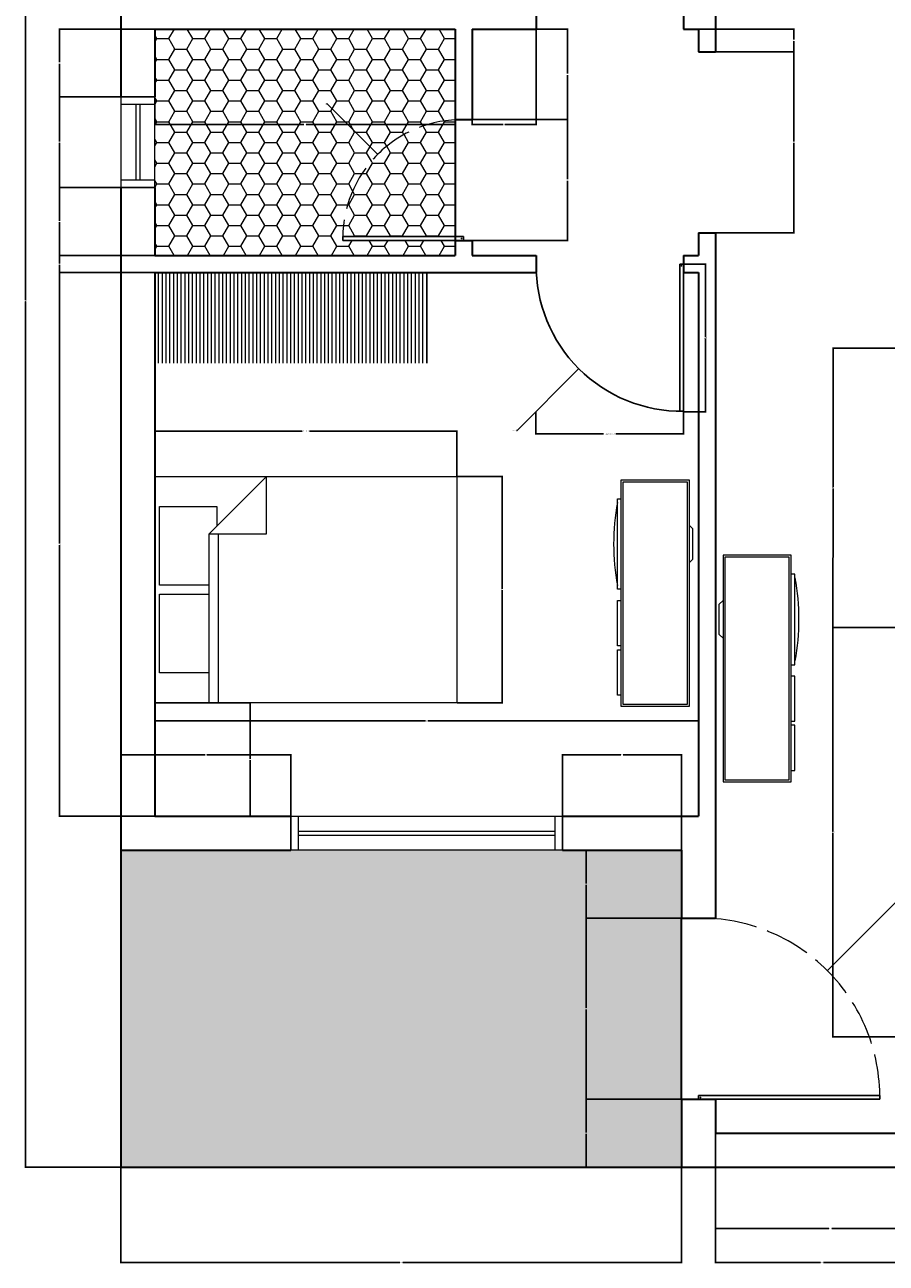
# Model space of a CAD drawing. Units: inches. Extents: x -1 to 436, y -13 to 497.
# Tile 1 of 4: x -1 to 227, y -13 to 315. Entities that reach past the tile are written whole.
import ezdxf

# ---------------------------------------------------------------- set-up
doc = ezdxf.new("R2010")
doc.units = ezdxf.units.IN
doc.linetypes.add('ACAD_ISO02W100', pattern=[15, 12, -3])
for name, color, linetype, lineweight in [('A-ANNO-DIMS', 2, 'Continuous', 18), ('A-DOOR', 4, 'Continuous', 25), ('A-DOOR-SWNG', 4, 'ACAD_ISO02W100', 13), ('A-FLOR-CASE', 8, 'Continuous', 25), ('A-FLOR-CASE-PATT', 9, 'Continuous', 13), ('A-FLOR-PATT', 9, 'Continuous', 13), ('A-FURN', 8, 'Continuous', 18), ('A-GLAZ', 4, 'Continuous', 18), ('A-WALL', 7, 'Continuous', 35)]:
    doc.layers.add(name, color=color, linetype=linetype, lineweight=lineweight)
doc.styles.get("Standard").update_dxf_attribs({"font": 'arial.ttf'})
doc.dimstyles.get("Standard").update_dxf_attribs({"dimtxt": 0.18, "dimasz": 0.18, "dimexe": 0.18, "dimexo": 0.0625, "dimgap": 0.09, "dimtad": 0, "dimtih": 1, "dimtoh": 1, "dimdec": 4, "dimzin": 0, "dimdsep": 46, "dimtxsty": 'Standard', "dimcen": 0.09, "dimadec": 0, "dimazin": 0, "dimtfac": 1, "dimtdec": 4, "dimtofl": 0, "dimtmove": 0, "dimatfit": 3, "dimfxl": 1, "dimtolj": 1, "dimtzin": 0, "dimarcsym": 0})
pattern_1 = [(0, (24, -128.4669), (4.7625, 2.74963), [3.175, -6.35]), (120, (24, -128.4669), (-4.7625, 2.74963), [3.175, -6.35]), (60, (24, -128.4669), (1e-08, 5.499261), [-6.35, 3.175])]

# ---------------------------------------------------------------- blocks, each defined once
blk = doc.blocks.new('Bed - Queen')
for p, q in [((0, -80.00003), (0, 0)), ((0, 0), (59.99999, 0)), ((59.99999, 0), (59.99999, -80.00003)), ((7.99999, -1.2), (28.79998, -1.2)), ((7.99999, -14.4), (7.99999, -1.2)), ((28.79998, -1.2), (28.79998, -14.4)), ((31.19999, -1.2), (51.99999, -1.2)), ((31.19999, -14.4), (31.19999, -1.2)), ((51.99999, -1.2), (51.99999, -16.4)), ((0, -14.4), (44.8, -14.4)), ((59.99999, -29.6), (44.8, -14.4)), ((44.8, -14.4), (44.8, -29.6)), ((51.99999, -16.4), (46.79936, -16.4)), ((44.8, -16.8), (0, -16.8)), ((44.8, -29.6), (59.99999, -29.6)), ((59.99999, -80.00003), (0, -80.00003))]:
    blk.add_line(p, q)
blk = doc.blocks.new('Entertainment Center')
for p, q in [((-4, 0), (-5, -1)), ((4, 0), (-4, 0)), ((5, -1), (4, 0)), ((-17, -19), (-17, -1)), ((-17, -1), (43, -1)), ((-16.5, -18.5), (-16.5, -1.5)), ((-16.5, -1.5), (42.5, -1.5)), ((42.5, -1.5), (42.5, -18.5)), ((43, -1), (43, -19)), ((43, -19), (-17, -19)), ((42.5, -18.5), (-16.5, -18.5)), ((-12, -20), (-12, -19)), ((12, -19), (12, -20)), ((15, -20), (15, -19)), ((27, -19), (27, -20)), ((28, -20), (28, -19)), ((40, -19), (40, -20)), ((12, -20), (-12, -20)), ((27, -20), (15, -20)), ((40, -20), (28, -20))]:
    blk.add_line(p, q)
blk.add_arc((0, 40), 61, 259.6111, 280.3889)
blk = doc.blocks.new('DOOR-SGL-39')
for p, q in [((38, 0), (38, 39)), ((38, 39), (39, 39)), ((39, 39), (39, 0)), ((39, 0), (38, 0))]:
    blk.add_line(p, q)
blk.add_arc((38.5, 38.5), 38.5, 179.2559, 270.7441)
blk = doc.blocks.new('WIN-FIXED-72')
for p, q in [((2, 0), (2, 9)), ((70, 0), (70, 9)), ((2, 5), (70, 5)), ((2, 4), (70, 4))]:
    blk.add_line(p, q)
blk.add_lwpolyline([(0, 9), (72, 9), (72, 0), (0, 0)], close=True)
blk = doc.blocks.new('*D14')
at = {"layer": 'A-ANNO-DIMS', "color": 0, "lineweight": -2, "transparency": 16777216}
for p, q in [((33, 195.6), (33, 207.71)), ((33.18, 207.53), (72.01, 207.53)), ((112.82, 207.53), (73.99, 207.53)), ((113, 195.6), (113, 207.71))]:
    blk.add_line(p, q, dxfattribs=at)
at = {"layer": 'A-ANNO-DIMS', "color": 0, "transparency": 16777216}
for points in [[(33.18, 207.56), (33.18, 207.5), (33, 207.53)], [(112.82, 207.56), (112.82, 207.5), (113, 207.53)]]:
    blk.add_solid(points, dxfattribs=at)
at = {"layer": 'Defpoints', "color": 0, "transparency": 16777216}
for p in [(33, 207.53), (33, 195.53), (113, 195.53)]:
    blk.add_point(p, dxfattribs=at)
at = {"layer": 'A-ANNO-DIMS', "color": 0, "transparency": 16777216, "insert": (73, 207.53), "char_height": 0.18, "attachment_point": 5}
blk.add_mtext('\\A1;QUEEN BED 80', dxfattribs=at)
blk = doc.blocks.new('*D15')
at = {"layer": 'A-ANNO-DIMS', "color": 0, "lineweight": -2, "transparency": 16777216}
for p, q in [((113.06, 195.53), (125.18, 195.53)), ((125, 195.35), (125, 165.72)), ((125, 135.71), (125, 165.35)), ((113.06, 135.53), (125.18, 135.53))]:
    blk.add_line(p, q, dxfattribs=at)
at = {"layer": 'A-ANNO-DIMS', "color": 0, "transparency": 16777216}
for points in [[(124.97, 195.35), (125.03, 195.35), (125, 195.53)], [(124.97, 135.71), (125.03, 135.71), (125, 135.53)]]:
    blk.add_solid(points, dxfattribs=at)
at = {"layer": 'Defpoints', "color": 0, "transparency": 16777216}
for p in [(113, 195.53), (125, 195.53), (113, 135.53)]:
    blk.add_point(p, dxfattribs=at)
at = {"layer": 'A-ANNO-DIMS', "color": 0, "transparency": 16777216, "insert": (125, 165.53), "char_height": 0.18, "attachment_point": 5}
blk.add_mtext('\\A1;60', dxfattribs=at)
blk = doc.blocks.new('*D24')
at = {"layer": 'A-ANNO-DIMS', "color": 0, "lineweight": -2, "transparency": 16777216}
for p, q in [((133.87, 212.59), (133.87, 206.6)), ((173, 212.59), (173, 206.6)), ((134.05, 206.78), (151.81, 206.78)), ((172.82, 206.78), (155.05, 206.78))]:
    blk.add_line(p, q, dxfattribs=at)
at = {"layer": 'A-ANNO-DIMS', "color": 0, "transparency": 16777216}
for points in [[(134.05, 206.81), (134.05, 206.75), (133.87, 206.78)], [(172.82, 206.81), (172.82, 206.75), (173, 206.78)]]:
    blk.add_solid(points, dxfattribs=at)
at = {"layer": 'Defpoints', "color": 0, "transparency": 16777216}
for p in [(133.87, 212.65), (173, 212.65), (173, 206.78)]:
    blk.add_point(p, dxfattribs=at)
at = {"layer": 'A-ANNO-DIMS', "color": 0, "transparency": 16777216, "insert": (153.43, 206.78), "char_height": 0.18, "attachment_point": 5}
blk.add_mtext('\\A1;BEDROOM DOOR 39 TYP.', dxfattribs=at)
blk = doc.blocks.new('*D25')
at = {"layer": 'A-ANNO-DIMS', "color": 0, "lineweight": -2, "transparency": 16777216}
for p, q in [((173.06, 251.78), (179.05, 251.78)), ((178.87, 251.6), (178.87, 232.4)), ((178.87, 212.83), (178.87, 232.03)), ((173.06, 212.65), (179.05, 212.65))]:
    blk.add_line(p, q, dxfattribs=at)
at = {"layer": 'A-ANNO-DIMS', "color": 0, "transparency": 16777216}
for points in [[(178.84, 251.6), (178.9, 251.6), (178.87, 251.78)], [(178.84, 212.83), (178.9, 212.83), (178.87, 212.65)]]:
    blk.add_solid(points, dxfattribs=at)
at = {"layer": 'Defpoints', "color": 0, "transparency": 16777216}
for p in [(173, 251.78), (178.87, 251.78), (173, 212.65)]:
    blk.add_point(p, dxfattribs=at)
at = {"layer": 'A-ANNO-DIMS', "color": 0, "transparency": 16777216, "insert": (178.87, 232.22), "char_height": 0.18, "attachment_point": 5}
blk.add_mtext('\\A1;39 TYP.', dxfattribs=at)
blk = doc.blocks.new('*D29')
at = {"layer": 'A-ANNO-DIMS', "color": 0, "lineweight": -2, "transparency": 16777216}
for p, q in [((23.94, 471.53), (-1.43, 471.53)), ((-1.25, 471.35), (-1.25, 242.22)), ((-1.25, 12.71), (-1.25, 241.85)), ((23.94, 12.53), (-1.43, 12.53))]:
    blk.add_line(p, q, dxfattribs=at)
at = {"layer": 'A-ANNO-DIMS', "color": 0, "transparency": 16777216}
for points in [[(-1.28, 471.35), (-1.22, 471.35), (-1.25, 471.53)], [(-1.28, 12.71), (-1.22, 12.71), (-1.25, 12.53)]]:
    blk.add_solid(points, dxfattribs=at)
at = {"layer": 'Defpoints', "color": 0, "transparency": 16777216}
for p in [(-1.25, 471.53), (24, 471.53), (24, 12.53)]:
    blk.add_point(p, dxfattribs=at)
at = {"layer": 'A-ANNO-DIMS', "color": 0, "transparency": 16777216, "insert": (-1.25, 242.03), "char_height": 0.18, "attachment_point": 5}
blk.add_mtext('\\A1;459', dxfattribs=at)
blk = doc.blocks.new('*D30')
at = {"layer": 'A-ANNO-DIMS', "color": 0, "lineweight": -2, "transparency": 16777216}
for p, q in [((181.5, 21.47), (181.5, -3.9)), ((242.25, 21.47), (242.25, -3.9)), ((181.68, -3.72), (211.48, -3.72)), ((242.07, -3.72), (212.27, -3.72))]:
    blk.add_line(p, q, dxfattribs=at)
at = {"layer": 'A-ANNO-DIMS', "color": 0, "transparency": 16777216}
for points in [[(181.68, -3.69), (181.68, -3.75), (181.5, -3.72)], [(242.07, -3.69), (242.07, -3.75), (242.25, -3.72)]]:
    blk.add_solid(points, dxfattribs=at)
at = {"layer": 'Defpoints', "color": 0, "transparency": 16777216}
for p in [(181.5, 21.53), (242.25, 21.53), (181.5, -3.72)]:
    blk.add_point(p, dxfattribs=at)
at = {"layer": 'A-ANNO-DIMS', "color": 0, "transparency": 16777216, "insert": (211.88, -3.72), "char_height": 0.18, "attachment_point": 5}
blk.add_mtext('\\A1;60.75', dxfattribs=at)
blk = doc.blocks.new('*D31')
at = {"layer": 'A-ANNO-DIMS', "color": 0, "lineweight": -2, "transparency": 16777216}
for p, q in [((24, 12.47), (24, -12.9)), ((172.5, 12.47), (172.5, -12.9)), ((24.18, -12.72), (97.86, -12.72)), ((172.32, -12.72), (98.64, -12.72))]:
    blk.add_line(p, q, dxfattribs=at)
at = {"layer": 'A-ANNO-DIMS', "color": 0, "transparency": 16777216}
for points in [[(24.18, -12.69), (24.18, -12.75), (24, -12.72)], [(172.32, -12.69), (172.32, -12.75), (172.5, -12.72)]]:
    blk.add_solid(points, dxfattribs=at)
at = {"layer": 'Defpoints', "color": 0, "transparency": 16777216}
for p in [(24, 12.53), (172.5, 12.53), (172.5, -12.72)]:
    blk.add_point(p, dxfattribs=at)
at = {"layer": 'A-ANNO-DIMS', "color": 0, "transparency": 16777216, "insert": (98.25, -12.72), "char_height": 0.18, "attachment_point": 5}
blk.add_mtext('\\A1;148.5', dxfattribs=at)
blk = doc.blocks.new('*D44')
at = {"layer": 'A-ANNO-DIMS', "color": 0, "lineweight": -2, "transparency": 16777216}
for p, q in [((32.94, 249.53), (7.57, 249.53)), ((7.75, 249.35), (7.75, 177.71)), ((7.75, 105.71), (7.75, 177.35)), ((32.94, 105.53), (7.57, 105.53))]:
    blk.add_line(p, q, dxfattribs=at)
at = {"layer": 'A-ANNO-DIMS', "color": 0, "transparency": 16777216}
for points in [[(7.72, 249.35), (7.78, 249.35), (7.75, 249.53)], [(7.72, 105.71), (7.78, 105.71), (7.75, 105.53)]]:
    blk.add_solid(points, dxfattribs=at)
at = {"layer": 'Defpoints', "color": 0, "transparency": 16777216}
for p in [(7.75, 249.53), (33, 249.53), (33, 105.53)]:
    blk.add_point(p, dxfattribs=at)
at = {"layer": 'A-ANNO-DIMS', "color": 0, "transparency": 16777216, "insert": (7.75, 177.53), "char_height": 0.18, "attachment_point": 5}
blk.add_mtext('\\A1;144', dxfattribs=at)
blk = doc.blocks.new('*D45')
at = {"layer": 'A-ANNO-DIMS', "color": 0, "lineweight": -2, "transparency": 16777216}
for p, q in [((32.94, 254.03), (7.57, 254.03)), ((7.75, 253.85), (7.75, 251.96)), ((32.94, 249.53), (7.57, 249.53)), ((7.75, 249.71), (7.75, 251.6))]:
    blk.add_line(p, q, dxfattribs=at)
at = {"layer": 'A-ANNO-DIMS', "color": 0, "transparency": 16777216}
for points in [[(7.72, 253.85), (7.78, 253.85), (7.75, 254.03)], [(7.72, 249.71), (7.78, 249.71), (7.75, 249.53)]]:
    blk.add_solid(points, dxfattribs=at)
at = {"layer": 'Defpoints', "color": 0, "transparency": 16777216}
for p in [(7.75, 254.03), (33, 254.03), (33, 249.53)]:
    blk.add_point(p, dxfattribs=at)
at = {"layer": 'A-ANNO-DIMS', "color": 0, "transparency": 16777216, "insert": (7.75, 251.78), "char_height": 0.18, "attachment_point": 5}
blk.add_mtext('\\A1;4.5', dxfattribs=at)
blk = doc.blocks.new('*D46')
at = {"layer": 'A-ANNO-DIMS', "color": 0, "lineweight": -2, "transparency": 16777216}
for p, q in [((32.94, 272.03), (7.57, 272.03)), ((7.75, 271.85), (7.75, 263.22)), ((7.75, 254.21), (7.75, 262.85)), ((32.94, 254.03), (7.57, 254.03))]:
    blk.add_line(p, q, dxfattribs=at)
at = {"layer": 'A-ANNO-DIMS', "color": 0, "transparency": 16777216}
for points in [[(7.72, 271.85), (7.78, 271.85), (7.75, 272.03)], [(7.72, 254.21), (7.78, 254.21), (7.75, 254.03)]]:
    blk.add_solid(points, dxfattribs=at)
at = {"layer": 'Defpoints', "color": 0, "transparency": 16777216}
for p in [(7.75, 272.03), (33, 272.03), (33, 254.03)]:
    blk.add_point(p, dxfattribs=at)
at = {"layer": 'A-ANNO-DIMS', "color": 0, "transparency": 16777216, "insert": (7.75, 263.03), "char_height": 0.18, "attachment_point": 5}
blk.add_mtext('\\A1;18', dxfattribs=at)
blk = doc.blocks.new('*D47')
at = {"layer": 'A-ANNO-DIMS', "color": 0, "lineweight": -2, "transparency": 16777216}
for p, q in [((32.94, 296.03), (7.57, 296.03)), ((7.75, 295.85), (7.75, 284.21)), ((7.75, 272.21), (7.75, 283.85)), ((32.94, 272.03), (7.57, 272.03))]:
    blk.add_line(p, q, dxfattribs=at)
at = {"layer": 'A-ANNO-DIMS', "color": 0, "transparency": 16777216}
for points in [[(7.72, 295.85), (7.78, 295.85), (7.75, 296.03)], [(7.72, 272.21), (7.78, 272.21), (7.75, 272.03)]]:
    blk.add_solid(points, dxfattribs=at)
at = {"layer": 'Defpoints', "color": 0, "transparency": 16777216}
for p in [(7.75, 296.03), (33, 296.03), (33, 272.03)]:
    blk.add_point(p, dxfattribs=at)
at = {"layer": 'A-ANNO-DIMS', "color": 0, "transparency": 16777216, "insert": (7.75, 284.03), "char_height": 0.18, "attachment_point": 5}
blk.add_mtext('\\A1;24', dxfattribs=at)
blk = doc.blocks.new('*D48')
at = {"layer": 'A-ANNO-DIMS', "color": 0, "lineweight": -2, "transparency": 16777216}
for p, q in [((32.94, 314.03), (7.57, 314.03)), ((7.75, 313.85), (7.75, 305.22)), ((7.75, 296.21), (7.75, 304.85)), ((32.94, 296.03), (7.57, 296.03))]:
    blk.add_line(p, q, dxfattribs=at)
at = {"layer": 'A-ANNO-DIMS', "color": 0, "transparency": 16777216}
for points in [[(7.72, 313.85), (7.78, 313.85), (7.75, 314.03)], [(7.72, 296.21), (7.78, 296.21), (7.75, 296.03)]]:
    blk.add_solid(points, dxfattribs=at)
at = {"layer": 'Defpoints', "color": 0, "transparency": 16777216}
for p in [(7.75, 314.03), (33, 314.03), (33, 296.03)]:
    blk.add_point(p, dxfattribs=at)
at = {"layer": 'A-ANNO-DIMS', "color": 0, "transparency": 16777216, "insert": (7.75, 305.03), "char_height": 0.18, "attachment_point": 5}
blk.add_mtext('\\A1;18', dxfattribs=at)
blk = doc.blocks.new('*D50')
at = {"layer": 'A-ANNO-DIMS', "color": 0, "lineweight": -2, "transparency": 16777216}
for p, q in [((24, 96.6), (24, 121.96)), ((24.18, 121.78), (46.28, 121.78)), ((68.82, 121.78), (46.72, 121.78)), ((69, 96.6), (69, 121.96))]:
    blk.add_line(p, q, dxfattribs=at)
at = {"layer": 'A-ANNO-DIMS', "color": 0, "transparency": 16777216}
for points in [[(24.18, 121.81), (24.18, 121.75), (24, 121.78)], [(68.82, 121.81), (68.82, 121.75), (69, 121.78)]]:
    blk.add_solid(points, dxfattribs=at)
at = {"layer": 'Defpoints', "color": 0, "transparency": 16777216}
for p in [(69, 121.78), (24, 96.53), (69, 96.53)]:
    blk.add_point(p, dxfattribs=at)
at = {"layer": 'A-ANNO-DIMS', "color": 0, "transparency": 16777216, "insert": (46.5, 121.78), "char_height": 0.18, "attachment_point": 5}
blk.add_mtext('\\A1;45', dxfattribs=at)
blk = doc.blocks.new('*D51')
at = {"layer": 'A-ANNO-DIMS', "color": 0, "lineweight": -2, "transparency": 16777216}
for p, q in [((141, 96.6), (141, 121.96)), ((141.18, 121.78), (156.43, 121.78)), ((172.32, 121.78), (157.07, 121.78)), ((172.5, 96.6), (172.5, 121.96))]:
    blk.add_line(p, q, dxfattribs=at)
at = {"layer": 'A-ANNO-DIMS', "color": 0, "transparency": 16777216}
for points in [[(141.18, 121.81), (141.18, 121.75), (141, 121.78)], [(172.32, 121.81), (172.32, 121.75), (172.5, 121.78)]]:
    blk.add_solid(points, dxfattribs=at)
at = {"layer": 'Defpoints', "color": 0, "transparency": 16777216}
for p in [(172.5, 121.78), (141, 96.53), (172.5, 96.53)]:
    blk.add_point(p, dxfattribs=at)
at = {"layer": 'A-ANNO-DIMS', "color": 0, "transparency": 16777216, "insert": (156.75, 121.78), "char_height": 0.18, "attachment_point": 5}
blk.add_mtext('\\A1;31.5', dxfattribs=at)
blk = doc.blocks.new('*D52')
at = {"layer": 'A-ANNO-DIMS', "color": 0, "lineweight": -2, "transparency": 16777216}
for p, q in [((33, 105.6), (33, 130.96)), ((33.18, 130.78), (104.72, 130.78)), ((176.82, 130.78), (105.28, 130.78)), ((177, 105.6), (177, 130.96))]:
    blk.add_line(p, q, dxfattribs=at)
at = {"layer": 'A-ANNO-DIMS', "color": 0, "transparency": 16777216}
for points in [[(33.18, 130.81), (33.18, 130.75), (33, 130.78)], [(176.82, 130.81), (176.82, 130.75), (177, 130.78)]]:
    blk.add_solid(points, dxfattribs=at)
at = {"layer": 'Defpoints', "color": 0, "transparency": 16777216}
for p in [(177, 130.78), (33, 105.53), (177, 105.53)]:
    blk.add_point(p, dxfattribs=at)
at = {"layer": 'A-ANNO-DIMS', "color": 0, "transparency": 16777216, "insert": (105, 130.78), "char_height": 0.18, "attachment_point": 5}
blk.add_mtext('\\A1;144', dxfattribs=at)
blk = doc.blocks.new('*D53')
at = {"layer": 'A-ANNO-DIMS', "color": 0, "lineweight": -2, "transparency": 16777216}
for p, q in [((33, 313.97), (33, 288.6)), ((112.5, 313.97), (112.5, 288.6)), ((33.18, 288.78), (72.43, 288.78)), ((112.32, 288.78), (73.07, 288.78))]:
    blk.add_line(p, q, dxfattribs=at)
at = {"layer": 'A-ANNO-DIMS', "color": 0, "transparency": 16777216}
for points in [[(33.18, 288.81), (33.18, 288.75), (33, 288.78)], [(112.32, 288.81), (112.32, 288.75), (112.5, 288.78)]]:
    blk.add_solid(points, dxfattribs=at)
at = {"layer": 'Defpoints', "color": 0, "transparency": 16777216}
for p in [(33, 314.03), (112.5, 314.03), (33, 288.78)]:
    blk.add_point(p, dxfattribs=at)
at = {"layer": 'A-ANNO-DIMS', "color": 0, "transparency": 16777216, "insert": (72.75, 288.78), "char_height": 0.18, "attachment_point": 5}
blk.add_mtext('\\A1;79.5', dxfattribs=at)
blk = doc.blocks.new('*D54')
at = {"layer": 'A-ANNO-DIMS', "color": 0, "lineweight": -2, "transparency": 16777216}
for p, q in [((117.06, 314.03), (142.43, 314.03)), ((142.25, 313.85), (142.25, 302.21)), ((142.25, 290.21), (142.25, 301.85)), ((117.06, 290.03), (142.43, 290.03))]:
    blk.add_line(p, q, dxfattribs=at)
at = {"layer": 'A-ANNO-DIMS', "color": 0, "transparency": 16777216}
for points in [[(142.22, 313.85), (142.28, 313.85), (142.25, 314.03)], [(142.22, 290.21), (142.28, 290.21), (142.25, 290.03)]]:
    blk.add_solid(points, dxfattribs=at)
at = {"layer": 'Defpoints', "color": 0, "transparency": 16777216}
for p in [(117, 314.03), (117, 290.03), (142.25, 290.03)]:
    blk.add_point(p, dxfattribs=at)
at = {"layer": 'A-ANNO-DIMS', "color": 0, "transparency": 16777216, "insert": (142.25, 302.03), "char_height": 0.18, "attachment_point": 5}
blk.add_mtext('\\A1;24', dxfattribs=at)
blk = doc.blocks.new('*D55')
at = {"layer": 'A-ANNO-DIMS', "color": 0, "lineweight": -2, "transparency": 16777216}
for p, q in [((117.06, 290.03), (142.43, 290.03)), ((142.25, 289.85), (142.25, 274.22)), ((142.25, 258.21), (142.25, 273.85)), ((117.06, 258.03), (142.43, 258.03))]:
    blk.add_line(p, q, dxfattribs=at)
at = {"layer": 'A-ANNO-DIMS', "color": 0, "transparency": 16777216}
for points in [[(142.22, 289.85), (142.28, 289.85), (142.25, 290.03)], [(142.22, 258.21), (142.28, 258.21), (142.25, 258.03)]]:
    blk.add_solid(points, dxfattribs=at)
at = {"layer": 'Defpoints', "color": 0, "transparency": 16777216}
for p in [(117, 290.03), (117, 258.03), (142.25, 258.03)]:
    blk.add_point(p, dxfattribs=at)
at = {"layer": 'A-ANNO-DIMS', "color": 0, "transparency": 16777216, "insert": (142.25, 274.03), "char_height": 0.18, "attachment_point": 5}
blk.add_mtext('\\A1;32', dxfattribs=at)
blk = doc.blocks.new('*D56')
at = {"layer": 'A-ANNO-DIMS', "color": 0, "lineweight": -2, "transparency": 16777216}
for p, q in [((117, 313.97), (117, 288.6)), ((134, 313.97), (134, 288.6)), ((117.18, 288.78), (125.29, 288.78)), ((133.82, 288.78), (125.71, 288.78))]:
    blk.add_line(p, q, dxfattribs=at)
at = {"layer": 'A-ANNO-DIMS', "color": 0, "transparency": 16777216}
for points in [[(117.18, 288.81), (117.18, 288.75), (117, 288.78)], [(133.82, 288.81), (133.82, 288.75), (134, 288.78)]]:
    blk.add_solid(points, dxfattribs=at)
at = {"layer": 'Defpoints', "color": 0, "transparency": 16777216}
for p in [(117, 314.03), (134, 314.03), (117, 288.78)]:
    blk.add_point(p, dxfattribs=at)
at = {"layer": 'A-ANNO-DIMS', "color": 0, "transparency": 16777216, "insert": (125.5, 288.78), "char_height": 0.18, "attachment_point": 5}
blk.add_mtext('\\A1;17', dxfattribs=at)
blk = doc.blocks.new('*D57')
at = {"layer": 'A-ANNO-DIMS', "color": 0, "lineweight": -2, "transparency": 16777216}
for p, q in [((177.06, 308.03), (202.43, 308.03)), ((202.25, 307.85), (202.25, 284.22)), ((202.25, 260.21), (202.25, 283.85)), ((177.06, 260.03), (202.43, 260.03))]:
    blk.add_line(p, q, dxfattribs=at)
at = {"layer": 'A-ANNO-DIMS', "color": 0, "transparency": 16777216}
for points in [[(202.22, 307.85), (202.28, 307.85), (202.25, 308.03)], [(202.22, 260.21), (202.28, 260.21), (202.25, 260.03)]]:
    blk.add_solid(points, dxfattribs=at)
at = {"layer": 'Defpoints', "color": 0, "transparency": 16777216}
for p in [(177, 308.03), (177, 260.03), (202.25, 260.03)]:
    blk.add_point(p, dxfattribs=at)
at = {"layer": 'A-ANNO-DIMS', "color": 0, "transparency": 16777216, "insert": (202.25, 284.03), "char_height": 0.18, "attachment_point": 5}
blk.add_mtext('\\A1;48', dxfattribs=at)
blk = doc.blocks.new('*D58')
at = {"layer": 'A-ANNO-DIMS', "color": 0, "lineweight": -2, "transparency": 16777216}
for p, q in [((177.06, 314.03), (202.43, 314.03)), ((202.25, 313.85), (202.25, 311.22)), ((202.25, 308.21), (202.25, 310.85)), ((177.06, 308.03), (202.43, 308.03))]:
    blk.add_line(p, q, dxfattribs=at)
at = {"layer": 'A-ANNO-DIMS', "color": 0, "transparency": 16777216}
for points in [[(202.22, 313.85), (202.28, 313.85), (202.25, 314.03)], [(202.22, 308.21), (202.28, 308.21), (202.25, 308.03)]]:
    blk.add_solid(points, dxfattribs=at)
at = {"layer": 'Defpoints', "color": 0, "transparency": 16777216}
for p in [(177, 314.03), (177, 308.03), (202.25, 308.03)]:
    blk.add_point(p, dxfattribs=at)
at = {"layer": 'A-ANNO-DIMS', "color": 0, "transparency": 16777216, "insert": (202.25, 311.03), "char_height": 0.18, "attachment_point": 5}
blk.add_mtext('\\A1;6', dxfattribs=at)
blk = doc.blocks.new('*D59')
at = {"layer": 'A-ANNO-DIMS', "color": 0, "lineweight": -2, "transparency": 16777216}
for p, q in [((172.44, 30.53), (147.07, 30.53)), ((147.25, 30.35), (147.25, 21.72)), ((147.25, 12.71), (147.25, 21.35)), ((172.44, 12.53), (147.07, 12.53))]:
    blk.add_line(p, q, dxfattribs=at)
at = {"layer": 'A-ANNO-DIMS', "color": 0, "transparency": 16777216}
for points in [[(147.22, 30.35), (147.28, 30.35), (147.25, 30.53)], [(147.22, 12.71), (147.28, 12.71), (147.25, 12.53)]]:
    blk.add_solid(points, dxfattribs=at)
at = {"layer": 'Defpoints', "color": 0, "transparency": 16777216}
for p in [(147.25, 30.53), (172.5, 30.53), (172.5, 12.53)]:
    blk.add_point(p, dxfattribs=at)
at = {"layer": 'A-ANNO-DIMS', "color": 0, "transparency": 16777216, "insert": (147.25, 21.53), "char_height": 0.18, "attachment_point": 5}
blk.add_mtext('\\A1;18', dxfattribs=at)
blk = doc.blocks.new('*D60')
at = {"layer": 'A-ANNO-DIMS', "color": 0, "lineweight": -2, "transparency": 16777216}
for p, q in [((172.44, 78.53), (147.07, 78.53)), ((147.25, 78.35), (147.25, 54.72)), ((147.25, 30.71), (147.25, 54.35)), ((172.44, 30.53), (147.07, 30.53))]:
    blk.add_line(p, q, dxfattribs=at)
at = {"layer": 'A-ANNO-DIMS', "color": 0, "transparency": 16777216}
for points in [[(147.22, 78.35), (147.28, 78.35), (147.25, 78.53)], [(147.22, 30.71), (147.28, 30.71), (147.25, 30.53)]]:
    blk.add_solid(points, dxfattribs=at)
at = {"layer": 'Defpoints', "color": 0, "transparency": 16777216}
for p in [(147.25, 78.53), (172.5, 78.53), (172.5, 30.53)]:
    blk.add_point(p, dxfattribs=at)
at = {"layer": 'A-ANNO-DIMS', "color": 0, "transparency": 16777216, "insert": (147.25, 54.53), "char_height": 0.18, "attachment_point": 5}
blk.add_mtext('\\A1;48', dxfattribs=at)
blk = doc.blocks.new('*D61')
at = {"layer": 'A-ANNO-DIMS', "color": 0, "lineweight": -2, "transparency": 16777216}
for p, q in [((172.44, 96.53), (147.07, 96.53)), ((147.25, 96.35), (147.25, 87.72)), ((147.25, 78.71), (147.25, 87.35)), ((172.44, 78.53), (147.07, 78.53))]:
    blk.add_line(p, q, dxfattribs=at)
at = {"layer": 'A-ANNO-DIMS', "color": 0, "transparency": 16777216}
for points in [[(147.22, 96.35), (147.28, 96.35), (147.25, 96.53)], [(147.22, 78.71), (147.28, 78.71), (147.25, 78.53)]]:
    blk.add_solid(points, dxfattribs=at)
at = {"layer": 'Defpoints', "color": 0, "transparency": 16777216}
for p in [(147.25, 96.53), (172.5, 96.53), (172.5, 78.53)]:
    blk.add_point(p, dxfattribs=at)
at = {"layer": 'A-ANNO-DIMS', "color": 0, "transparency": 16777216, "insert": (147.25, 87.53), "char_height": 0.18, "attachment_point": 5}
blk.add_mtext('\\A1;18', dxfattribs=at)
blk = doc.blocks.new('*D65')
at = {"layer": 'A-ANNO-DIMS', "color": 0, "lineweight": -2, "transparency": 16777216}
for p, q in [((33.06, 135.53), (58.43, 135.53)), ((58.25, 135.35), (58.25, 120.72)), ((58.25, 105.71), (58.25, 120.35)), ((33.06, 105.53), (58.43, 105.53))]:
    blk.add_line(p, q, dxfattribs=at)
at = {"layer": 'A-ANNO-DIMS', "color": 0, "transparency": 16777216}
for points in [[(58.22, 135.35), (58.28, 135.35), (58.25, 135.53)], [(58.22, 105.71), (58.28, 105.71), (58.25, 105.53)]]:
    blk.add_solid(points, dxfattribs=at)
at = {"layer": 'Defpoints', "color": 0, "transparency": 16777216}
for p in [(33, 135.53), (33, 105.53), (58.25, 105.53)]:
    blk.add_point(p, dxfattribs=at)
at = {"layer": 'A-ANNO-DIMS', "color": 0, "transparency": 16777216, "insert": (58.25, 120.53), "char_height": 0.18, "attachment_point": 5}
blk.add_mtext('\\A1;30', dxfattribs=at)
blk = doc.blocks.new('*D70')
at = {"layer": 'A-ANNO-DIMS', "color": 0, "lineweight": -2, "transparency": 16777216}
for p, q in [((237.77, 155.49), (212.4, 155.49)), ((212.58, 155.31), (212.58, 101.48)), ((212.58, 47.29), (212.58, 101.11)), ((237.77, 47.11), (212.4, 47.11))]:
    blk.add_line(p, q, dxfattribs=at)
at = {"layer": 'A-ANNO-DIMS', "color": 0, "transparency": 16777216}
for points in [[(212.55, 155.31), (212.61, 155.31), (212.58, 155.49)], [(212.55, 47.29), (212.61, 47.29), (212.58, 47.11)]]:
    blk.add_solid(points, dxfattribs=at)
at = {"layer": 'Defpoints', "color": 0, "transparency": 16777216}
for p in [(212.58, 155.49), (237.83, 155.49), (237.83, 47.11)]:
    blk.add_point(p, dxfattribs=at)
at = {"layer": 'A-ANNO-DIMS', "color": 0, "transparency": 16777216, "insert": (212.58, 101.3), "char_height": 0.18, "attachment_point": 5}
blk.add_mtext('\\A1;108.38', dxfattribs=at)
blk = doc.blocks.new('*D72')
at = {"layer": 'A-ANNO-DIMS', "color": 0, "lineweight": -2, "transparency": 16777216}
for p, q in [((237.83, 229.51), (212.46, 229.53)), ((212.64, 229.35), (212.61, 192.7)), ((212.58, 155.69), (212.61, 192.34)), ((237.77, 155.49), (212.4, 155.51))]:
    blk.add_line(p, q, dxfattribs=at)
at = {"layer": 'A-ANNO-DIMS', "color": 0, "transparency": 16777216}
for points in [[(212.61, 229.35), (212.67, 229.35), (212.64, 229.53)], [(212.55, 155.69), (212.61, 155.69), (212.58, 155.51)]]:
    blk.add_solid(points, dxfattribs=at)
at = {"layer": 'Defpoints', "color": 0, "transparency": 16777216}
for p in [(212.64, 229.53), (237.89, 229.51), (237.83, 155.49)]:
    blk.add_point(p, dxfattribs=at)
at = {"layer": 'A-ANNO-DIMS', "color": 0, "transparency": 16777216, "insert": (212.61, 192.52), "char_height": 0.18, "attachment_point": 5}
blk.add_mtext('\\A1;74.03', dxfattribs=at)
blk = doc.blocks.new('*D77')
at = {"layer": 'A-ANNO-DIMS', "color": 0, "lineweight": -2, "transparency": 16777216}
for p, q in [((237.83, 47.04), (237.83, -12.9)), ((181.5, 21.47), (181.5, -12.9)), ((181.68, -12.72), (209.27, -12.72)), ((237.65, -12.72), (210.06, -12.72))]:
    blk.add_line(p, q, dxfattribs=at)
at = {"layer": 'A-ANNO-DIMS', "color": 0, "transparency": 16777216}
for points in [[(181.68, -12.69), (181.68, -12.75), (181.5, -12.72)], [(237.65, -12.69), (237.65, -12.75), (237.83, -12.72)]]:
    blk.add_solid(points, dxfattribs=at)
at = {"layer": 'Defpoints', "color": 0, "transparency": 16777216}
for p in [(237.83, 47.11), (181.5, 21.53), (237.83, -12.72)]:
    blk.add_point(p, dxfattribs=at)
at = {"layer": 'A-ANNO-DIMS', "color": 0, "transparency": 16777216, "insert": (209.67, -12.72), "char_height": 0.18, "attachment_point": 5}
blk.add_mtext('\\A1;56.33', dxfattribs=at)
blk = doc.blocks.new('*D83')
at = {"layer": 'A-ANNO-DIMS', "color": 0, "lineweight": -2, "transparency": 16777216}
for p, q in [((231.24, 84.78), (211.22, 64.75)), ((231.42, 84.78), (231.24, 84.78)), ((177.41, 31.03), (177.59, 31.03)), ((177.5, 30.94), (177.5, 31.12))]:
    blk.add_line(p, q, dxfattribs=at)
at = {"layer": 'A-ANNO-DIMS', "color": 0, "transparency": 16777216}
blk.add_solid([(211.2, 64.77), (211.24, 64.73), (211.09, 64.62)], dxfattribs=at)
at = {"layer": 'Defpoints', "color": 0, "transparency": 16777216}
for p in [(211.09, 64.62), (177.5, 31.03)]:
    blk.add_point(p, dxfattribs=at)
at = {"layer": 'A-ANNO-DIMS', "color": 0, "transparency": 16777216, "insert": (231.83, 84.78), "char_height": 0.18, "attachment_point": 5}
blk.add_mtext('\\A1;R47.5', dxfattribs=at)
blk = doc.blocks.new('*D84')
at = {"layer": 'A-ANNO-DIMS', "color": 0, "lineweight": -2, "transparency": 16777216}
for p, q in [((172.41, 251.28), (172.59, 251.28)), ((172.5, 251.19), (172.5, 251.37)), ((128.94, 207.72), (145.15, 223.93)), ((128.76, 207.72), (128.94, 207.72))]:
    blk.add_line(p, q, dxfattribs=at)
at = {"layer": 'A-ANNO-DIMS', "color": 0, "transparency": 16777216}
blk.add_solid([(145.13, 223.95), (145.17, 223.91), (145.27, 224.06)], dxfattribs=at)
at = {"layer": 'Defpoints', "color": 0, "transparency": 16777216}
for p in [(172.5, 251.28), (145.27, 224.06)]:
    blk.add_point(p, dxfattribs=at)
at = {"layer": 'A-ANNO-DIMS', "color": 0, "transparency": 16777216, "insert": (128.15, 207.72), "char_height": 0.18, "attachment_point": 5}
blk.add_mtext('\\A1;2X R38.5', dxfattribs=at)
blk = doc.blocks.new('*D85')
at = {"layer": 'A-ANNO-DIMS', "color": 0, "lineweight": -2, "transparency": 16777216}
for p, q in [((78.43, 294.18), (78.61, 294.18)), ((78.61, 294.18), (91.85, 280.94)), ((114.16, 258.53), (114.34, 258.53)), ((114.25, 258.44), (114.25, 258.62))]:
    blk.add_line(p, q, dxfattribs=at)
at = {"layer": 'A-ANNO-DIMS', "color": 0, "transparency": 16777216}
blk.add_solid([(91.87, 280.96), (91.82, 280.92), (91.97, 280.81)], dxfattribs=at)
at = {"layer": 'Defpoints', "color": 0, "transparency": 16777216}
for p in [(91.97, 280.81), (114.25, 258.53)]:
    blk.add_point(p, dxfattribs=at)
at = {"layer": 'A-ANNO-DIMS', "color": 0, "transparency": 16777216, "insert": (77.88, 294.18), "char_height": 0.18, "attachment_point": 5}
blk.add_mtext('\\A1;R31.504', dxfattribs=at)

msp = doc.modelspace()

# ---------------------------------------------------------------- hatches: boundary and pattern name
at = {"layer": 'A-FLOR-CASE-PATT'}
h = msp.add_hatch(dxfattribs=at)
h.set_pattern_fill('ANSI31', color=256, scale=0.31496, angle=45, style=0)
h.paths.add_polyline_path([(33, 225.5331), (105, 225.5331), (105, 249.5331), (33, 249.5331)])
at = {"layer": 'A-FLOR-PATT'}
h = msp.add_hatch(dxfattribs=at)
h.set_pattern_fill('HONEY', color=256)
h.set_pattern_definition(pattern_1)
h.paths.add_polyline_path([(33, 272.0331), (33, 254.0331), (112.5, 254.0331), (112.5, 258.0331), (82.75, 258.0331, -0.40263134), (112.5, 289.9885), (112.5, 290.0331), (112.5, 314.0331), (33, 314.0331), (33, 296.0331)])
h = msp.add_hatch(dxfattribs=at)
h.set_pattern_fill('HONEY', color=256)
h.set_pattern_definition(pattern_1)
h.paths.add_polyline_path([(82.75, 259.0331), (112.5, 259.0331), (112.5, 289.9885, 0.39343818)])
h = msp.add_hatch(color=256, dxfattribs=at)
h.dxf.hatch_style = 1
h.paths.add_polyline_path([(69, 96.5331), (24, 96.5331), (24, 12.5331), (172.5, 12.5331), (172.5, 30.5331), (172.5, 78.5331), (172.5, 96.5331), (141, 96.5331)])

# ---------------------------------------------------------------- linework, layer by layer
at = {"layer": 'A-DOOR'}
for p, q in [((82.75, 258.0331), (82.75, 259.0331)), ((82.75, 259.0331), (114.75, 259.0331)), ((114.75, 258.0331), (82.75, 258.0331)), ((114.75, 259.0331), (114.75, 258.0331)), ((225, 31.5331), (177, 31.5331)), ((177, 31.5331), (177, 30.5331)), ((177, 30.5331), (225, 30.5331)), ((225, 30.5331), (225, 31.5331))]:
    msp.add_line(p, q, dxfattribs=at)
at = {"layer": 'A-DOOR-SWNG'}
for centre, radius, start, end in [((114.25, 258.5331), 31.504, 89.09062, 180.90938), ((177.5, 31.0331), 47.5026, 359.396909, 90.603091)]:
    msp.add_arc(centre, radius, start, end, dxfattribs=at)
at = {"layer": 'A-FLOR-CASE'}
for p, q in [((33, 249.5331), (105, 249.5331)), ((33, 249.5331), (33, 225.5331)), ((105, 249.5331), (105, 225.5331)), ((105, 245.474), (105, 249.5331))]:
    msp.add_line(p, q, dxfattribs=at)
at = {"layer": 'A-GLAZ'}
for p, q in [((24, 296.0331), (33, 296.0331)), ((33, 294.0331), (24, 294.0331)), ((28, 294.0331), (28, 274.0331)), ((29, 294.0331), (29, 274.0331)), ((33, 274.0331), (24, 274.0331)), ((33, 272.0331), (33, 274.0331)), ((24, 272.0331), (33, 272.0331)), ((69, 105.5331), (69, 96.5331)), ((69, 96.5331), (69, 105.5331)), ((141, 105.5331), (141, 96.5331))]:
    msp.add_line(p, q, dxfattribs=at)
msp.add_lwpolyline([(33, 296.0331), (24, 296.0331), (24, 272.0331), (33, 272.0331)], close=True, dxfattribs=at)
at = {"layer": 'A-WALL'}
for p, q in [((24, 471.5331), (24, 296.0331)), ((181.5, 390.5331), (181.5, 308.0331)), ((134, 318.5331), (134, 314.0331)), ((173, 318.5331), (173, 314.0331)), ((33, 314.0331), (112.5, 314.0331)), ((33, 314.0331), (33, 296.0331)), ((112.5, 314.0331), (112.5, 290.0331)), ((117, 314.0331), (117, 290.0331)), ((117, 314.0331), (134, 314.0331)), ((173, 314.0331), (177, 314.0331)), ((177, 314.0331), (177, 308.0331)), ((177, 308.0331), (181.5, 308.0331)), ((112.5, 290.0331), (117, 290.0331)), ((112.5, 290.0331), (112.5, 258.0331)), ((24, 272.0331), (24, 12.5331)), ((33, 272.0331), (33, 254.0331)), ((177, 260.0331), (177, 254.0331)), ((177, 260.0331), (181.5, 260.0331)), ((181.5, 260.0331), (181.5, 78.5331)), ((112.5, 258.0331), (117, 258.0331)), ((112.5, 258.0331), (112.5, 254.0331)), ((117, 258.0331), (117, 254.0331)), ((33, 254.0331), (112.5, 254.0331)), ((117, 254.0331), (134, 254.0331)), ((134, 254.0331), (134, 249.5331)), ((173, 254.0331), (173, 249.5331)), ((173, 254.0331), (177, 254.0331)), ((33, 249.5331), (134, 249.5331)), ((33, 249.5331), (33, 105.5331)), ((173, 249.5331), (177, 249.5331)), ((177, 249.5331), (177, 105.5331)), ((33, 105.5331), (69, 105.5331)), ((141, 105.5331), (177, 105.5331)), ((24, 96.5331), (69, 96.5331)), ((141, 96.5331), (172.5, 96.5331)), ((172.5, 96.5331), (172.5, 78.5331)), ((172.5, 78.5331), (181.5, 78.5331)), ((172.5, 30.5331), (172.5, 78.5331)), ((172.5, 30.5331), (181.5, 30.5331)), ((172.5, 30.5331), (172.5, 12.5331)), ((181.5, 30.5331), (181.5, 21.5331)), ((181.5, 21.5331), (375, 21.5331)), ((24, 12.5331), (177, 12.5331)), ((177, 12.5331), (384, 12.5331))]:
    msp.add_line(p, q, dxfattribs=at)

# ---------------------------------------------------------------- block references
at = {"layer": 'A-DOOR'}
msp.add_blockref('DOOR-SGL-39', (134, 212.783), dxfattribs=at)
at = {"layer": 'A-FURN'}
for name, p, rotation in [('Bed - Queen', (33, 135.5331), 90), ('Entertainment Center', (175.5046, 177.6167), 270)]:
    msp.add_blockref(name, p, dxfattribs=dict(at, rotation=rotation))
at = {"layer": 'A-FURN', "xscale": -1, "rotation": 90}
msp.add_blockref('Entertainment Center', (182.4965, 157.6506), dxfattribs=at)
at = {"layer": 'A-GLAZ'}
msp.add_blockref('WIN-FIXED-72', (69, 96.533), dxfattribs=at)

# ---------------------------------------------------------------- dimensions: what is measured, and where the dimension line sits
at = {"layer": 'A-ANNO-DIMS'}
for base, p1, p2, angle, override, picture, middle in [((-1.25, 471.5331), (24, 12.5331), (24, 471.5331), 90, {"dimdec": 0, "dimlfac": 1, "dimrnd": 0, "dimzin": 0, "dimdsep": 46, "dimlunit": 2}, '*D29', (-1.25, 242.0331)), ((7.75, 314.0331), (33, 296.0331), (33, 314.0331), 90, {"dimdec": 0, "dimlfac": 1, "dimrnd": 0, "dimzin": 0, "dimdsep": 46, "dimlunit": 2}, '*D48', (7.75, 305.0331)), ((33, 288.7831), (112.5, 314.0331), (33, 314.0331), 180, {"dimdec": 1, "dimlfac": 1, "dimrnd": 0, "dimzin": 0, "dimdsep": 46, "dimlunit": 2}, '*D53', (72.75, 288.7831)), ((142.25, 290.0331), (117, 314.0331), (117, 290.0331), 270, {"dimdec": 0, "dimlfac": 1, "dimrnd": 0, "dimzin": 0, "dimdsep": 46, "dimlunit": 2}, '*D54', (142.25, 302.0331)), ((117, 288.7831), (134, 314.0331), (117, 314.0331), 180, {"dimdec": 0, "dimlfac": 1, "dimrnd": 0, "dimzin": 0, "dimdsep": 46, "dimlunit": 2}, '*D56', (125.5, 288.7831)), ((202.25, 308.0331), (177, 314.0331), (177, 308.0331), 270, {"dimdec": 0, "dimlfac": 1, "dimrnd": 0, "dimzin": 0, "dimdsep": 46, "dimlunit": 2}, '*D58', (202.25, 311.0331)), ((202.25, 260.0331), (177, 308.0331), (177, 260.0331), 270, {"dimdec": 0, "dimlfac": 1, "dimrnd": 0, "dimzin": 0, "dimdsep": 46, "dimlunit": 2}, '*D57', (202.25, 284.0331)), ((7.75, 296.0331), (33, 272.0331), (33, 296.0331), 90, {"dimdec": 0, "dimlfac": 1, "dimrnd": 0, "dimzin": 0, "dimdsep": 46, "dimlunit": 2}, '*D47', (7.75, 284.0331)), ((142.25, 258.0331), (117, 290.0331), (117, 258.0331), 270, {"dimdec": 0, "dimlfac": 1, "dimrnd": 0, "dimzin": 0, "dimdsep": 46, "dimlunit": 2}, '*D55', (142.25, 274.0331)), ((7.75, 272.0331), (33, 254.0331), (33, 272.0331), 90, {"dimdec": 0, "dimlfac": 1, "dimrnd": 0, "dimzin": 0, "dimdsep": 46, "dimlunit": 2}, '*D46', (7.75, 263.0331)), ((7.75, 254.0331), (33, 249.5331), (33, 254.0331), 90, {"dimdec": 1, "dimlfac": 1, "dimrnd": 0, "dimzin": 0, "dimdsep": 46, "dimlunit": 2}, '*D45', (7.75, 251.7831)), ((7.75, 249.5331), (33, 105.5331), (33, 249.5331), 90, {"dimdec": 0, "dimlfac": 1, "dimrnd": 0, "dimzin": 0, "dimdsep": 46, "dimlunit": 2}, '*D44', (7.75, 177.5331)), ((212.6448, 229.5338), (237.8302, 155.4864), (237.8948, 229.5117), 89.949986, {"dimdec": 2, "dimlfac": 1, "dimrnd": 0, "dimzin": 0, "dimdsep": 46, "dimlunit": 2}, '*D72', (212.6125, 192.5211)), ((125, 195.5331), (113, 135.5331), (113, 195.5331), 90, {"dimdec": 0, "dimlfac": 1, "dimrnd": 0, "dimzin": 0, "dimdsep": 46, "dimlunit": 2}, '*D15', (125, 165.5331)), ((212.5802, 155.4864), (237.8302, 47.1064), (237.8302, 155.4864), 90, {"dimdec": 2, "dimlfac": 1, "dimrnd": 0, "dimzin": 0, "dimdsep": 46, "dimlunit": 2}, '*D70', (212.5802, 101.2964)), ((58.25, 105.5331), (33, 135.5331), (33, 105.5331), 270, {"dimdec": 0, "dimlfac": 1, "dimrnd": 0, "dimzin": 0, "dimdsep": 46, "dimlunit": 2}, '*D65', (58.25, 120.5331)), ((147.25, 96.5331), (172.5, 78.5331), (172.5, 96.5331), 90, {"dimdec": 0, "dimlfac": 1, "dimrnd": 0, "dimzin": 0, "dimdsep": 46, "dimlunit": 2}, '*D61', (147.25, 87.5331)), ((147.25, 78.5331), (172.5, 30.5331), (172.5, 78.5331), 90, {"dimdec": 0, "dimlfac": 1, "dimrnd": 0, "dimzin": 0, "dimdsep": 46, "dimlunit": 2}, '*D60', (147.25, 54.5331)), ((147.25, 30.5331), (172.5, 12.5331), (172.5, 30.5331), 90, {"dimdec": 0, "dimlfac": 1, "dimrnd": 0, "dimzin": 0, "dimdsep": 46, "dimlunit": 2}, '*D59', (147.25, 21.5331)), ((181.5, -3.7169), (242.25, 21.5331), (181.5, 21.5331), 180, {"dimdec": 2, "dimlfac": 1, "dimrnd": 0, "dimzin": 0, "dimdsep": 46, "dimlunit": 2}, '*D30', (211.875, -3.7169))]:
    dim = msp.add_linear_dim(base=base, p1=p1, p2=p2, angle=angle, dimstyle='Standard', override=override, dxfattribs=at)
    dim.commit()
    dim.dimension.update_dxf_attribs({"geometry": picture, "text_midpoint": middle})
for center, mpoint, override, picture, middle in [((114.25, 258.5331), (91.9733, 280.8097), {"dimdec": 3, "dimlfac": 1, "dimrnd": 0, "dimzin": 0, "dimdsep": 46, "dimlunit": 2}, '*D85', (77.8778, 294.1757)), ((177.5, 31.0331), (211.089, 64.623), {"dimdec": 1, "dimlfac": 1, "dimrnd": 0, "dimzin": 0, "dimdsep": 46, "dimlunit": 2}, '*D83', (231.833, 84.7769))]:
    dim = msp.add_radius_dim(center=center, mpoint=mpoint, dimstyle='Standard', override=override, dxfattribs=at)
    dim.commit()
    dim.dimension.update_dxf_attribs({"geometry": picture, "text_midpoint": middle, "dimtype": 164})
dim = msp.add_radius_dim(center=(172.5, 251.2831), mpoint=(145.2742, 224.0572), text='2X <>', dimstyle='Standard', override={"dimdec": 1, "dimlfac": 1, "dimrnd": 0, "dimzin": 0, "dimdsep": 46, "dimlunit": 2}, dxfattribs=at)
dim.commit()
dim.dimension.update_dxf_attribs({"geometry": '*D84', "text_midpoint": (128.1532, 207.7216), "dimtype": 164})
for base, p1, p2, angle, text, picture, middle in [((178.8702, 251.7831), (173, 212.6483), (173, 251.7831), 90, '<> TYP.', '*D25', (178.8702, 232.2157)), ((33, 207.5331), (113, 195.5331), (33, 195.5331), 180, 'QUEEN BED <>', '*D14', (73, 207.5331))]:
    dim = msp.add_linear_dim(base=base, p1=p1, p2=p2, angle=angle, text=text, dimstyle='Standard', override={"dimdec": 0, "dimlfac": 1, "dimrnd": 0, "dimzin": 0, "dimdsep": 46, "dimlunit": 2}, dxfattribs=at)
    dim.commit()
    dim.dimension.update_dxf_attribs({"geometry": picture, "text_midpoint": middle})
dim = msp.add_linear_dim(base=(173, 206.7781), p1=(133.8651, 212.6483), p2=(173, 212.6483), text='BEDROOM DOOR <> TYP.', dimstyle='Standard', override={"dimdec": 0, "dimlfac": 1, "dimrnd": 0, "dimzin": 0, "dimdsep": 46, "dimlunit": 2}, dxfattribs=at)
dim.commit()
dim.dimension.update_dxf_attribs({"geometry": '*D24', "text_midpoint": (153.4326, 206.7781)})
for base, p1, p2, override, picture, middle in [((177, 130.7831), (33, 105.5331), (177, 105.5331), {"dimdec": 0, "dimlfac": 1, "dimrnd": 0, "dimzin": 0, "dimdsep": 46, "dimlunit": 2}, '*D52', (105, 130.7831)), ((69, 121.7831), (24, 96.5331), (69, 96.5331), {"dimdec": 0, "dimlfac": 1, "dimrnd": 0, "dimzin": 0, "dimdsep": 46, "dimlunit": 2}, '*D50', (46.5, 121.7831)), ((172.5, 121.7831), (141, 96.5331), (172.5, 96.5331), {"dimdec": 1, "dimlfac": 1, "dimrnd": 0, "dimzin": 0, "dimdsep": 46, "dimlunit": 2}, '*D51', (156.75, 121.7831)), ((237.8302, -12.7169), (181.5, 21.5331), (237.8302, 47.1064), {"dimdec": 2, "dimlfac": 1, "dimrnd": 0, "dimzin": 0, "dimdsep": 46, "dimlunit": 2}, '*D77', (209.6651, -12.7169)), ((172.5, -12.7169), (24, 12.5331), (172.5, 12.5331), {"dimdec": 1, "dimlfac": 1, "dimrnd": 0, "dimzin": 0, "dimdsep": 46, "dimlunit": 2}, '*D31', (98.25, -12.7169))]:
    dim = msp.add_linear_dim(base=base, p1=p1, p2=p2, dimstyle='Standard', override=override, dxfattribs=at)
    dim.commit()
    dim.dimension.update_dxf_attribs({"geometry": picture, "text_midpoint": middle})

doc.saveas('drawing.dxf')
